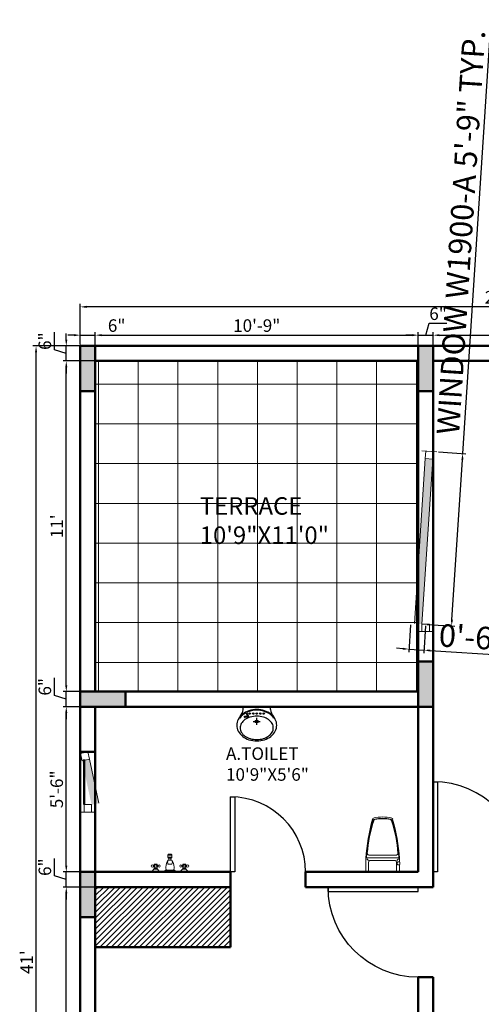
# Model space of a CAD drawing. Units: inches. Extents: x 3064 to 19385, y 846 to 15425.
# Tile 73 of 108: x 6445 to 6629, y 1725 to 2118. Entities that reach past the tile are written whole.
import ezdxf

# ---------------------------------------------------------------- set-up
doc = ezdxf.new("R2010")
doc.units = ezdxf.units.IN
for name, color, linetype, lineweight in [('A-ANNO-DIMS', 2, 'Continuous', 18), ('A-AREA-IDEN', 3, 'Continuous', 18), ('A-COLS', 1, 'Continuous', 35), ('A-DOOR', 3, 'Continuous', 25), ('A-FLOR-FIXT', 9, 'Continuous', 18), ('A-FLOR-PATT', 252, 'Continuous', 13), ('A-FURN-PATT', 252, 'Continuous', 13), ('A-GLAZ', 4, 'Continuous', 18), ('A-WALL', 7, 'Continuous', 50)]:
    doc.layers.add(name, color=color, linetype=linetype, lineweight=lineweight)
doc.layers.add('THIET-BI', color=21, linetype='Continuous')
doc.styles.get("Standard").update_dxf_attribs({"font": 'arial.ttf'})
doc.dimstyles.new('ISO-25', dxfattribs={"dimtxt": 9, "dimasz": 2.5, "dimexe": 1.25, "dimexo": 0.625, "dimtad": 1, "dimdec": 1, "dimlunit": 3, "dimtxsty": 'Standard', "dimcen": 2.5, "dimadec": 0, "dimazin": 0, "dimtfac": 1, "dimtdec": 1, "dimtmove": 0, "dimatfit": 3, "dimfxl": 1, "dimarcsym": 0})

# ---------------------------------------------------------------- blocks, each defined once
blk = doc.blocks.new('*U3')
for p, q in [((0, 0), (0, -6)), ((36, 0), (36, -6))]:
    blk.add_line(p, q)
blk.add_lwpolyline([(0, 0), (0, 36), (1.75, 36), (1.75, 0)], close=True)
blk.add_arc((0, 0), 36, 0, 90)
blk = doc.blocks.new('*U4')
for p, q in [((0, 0), (0, -6)), ((30, 0), (30, -6))]:
    blk.add_line(p, q)
blk.add_lwpolyline([(0, 0), (0, 30), (1.75, 30), (1.75, 0)], close=True)
blk.add_arc((0, 0), 30, 0, 90)
blk = doc.blocks.new('A$C430D11A0')
at = {"layer": 'THIET-BI'}
for p, q in [((90, 445), (90, 485)), ((475, 485), (90, 485)), ((475, 483), (90, 483)), ((475, 445), (475, 485)), ((129, 398), (158, 344)), ((138, 403), (176, 332)), ((282, 226), (282, 325)), ((233, 275), (332, 275))]:
    blk.add_line(p, q, dxfattribs=at)
for points in [[(565, 223, 0.121635), (545, 305, 0.10526), (482, 380, 0.088175), (393, 427, 0.079002), (282, 445, 0.079002), (172, 427, 0.088175), (83, 380, 0.10526), (20, 305, 0.121635), (0, 223, 0.121635), (20, 140, 0.10526), (83, 65, 0.088175), (172, 18, 0.079002), (282, 0, 0.079002), (393, 18, 0.088175), (482, 65, 0.10526), (545, 140, 0.121635)], [(517, 185, 0.134042), (501, 245, 0.106817), (449, 302, 0.082468), (376, 337, 0.070874), (282, 350, 0.070874), (189, 337, 0.082468), (116, 302, 0.106817), (64, 245, 0.134042), (47, 185, 0.134042), (64, 125, 0.106817), (116, 68, 0.082468), (189, 33, 0.070874), (282, 20, 0.070874), (376, 33, 0.082468), (449, 68, 0.106817), (501, 125, 0.134042)]]:
    blk.add_lwpolyline(points, format="xyb", close=True, dxfattribs=at)
for points in [[(523, 322, 0.07708), (476, 372, 0.088175), (390, 418, 0.079002), (282, 435, 0.079002), (175, 418, 0.035427), (138, 403, 0.07708)], [(129, 398, 0.043566), (89, 372, 0.07708), (42, 322, 0.041486)]]:
    blk.add_lwpolyline(points, format="xyb", dxfattribs=at)
for centre, radius in [((182, 388), 10.5), ((232, 388), 10.5), ((282, 275), 20), ((282, 275), 15), ((282, 388), 10.5), ((332, 388), 10.5), ((382, 388), 10.5)]:
    blk.add_circle(centre, radius, dxfattribs=at)
for centre, radius, start, end in [((-104, 469), 195, 320.8253, 352.9557), ((669, 469), 195, 187.0443, 219.1747), ((136, 285), 62.9, 69.643, 123.4774), ((136, 285), 52.9, 55.2455, 123.4774)]:
    blk.add_arc(centre, radius, start, end, dxfattribs=at)
blk = doc.blocks.new('WC-P05')
for p, q in [((-210, 430), (-210, 409)), ((-202, 532), (-202, 439)), ((-201, 439), (-180, 439)), ((-192, 542), (263, 542)), ((-171, 430), (-171, 409)), ((-163, 542), (-163, 401)), ((234, 542), (234, 401)), ((273, 532), (273, 352)), ((-202, 400), (-202, 352)), ((-201, 400), (-180, 400)), ((-192, 342), (263, 342)), ((-167, 379), (-188, 357)), ((-159, 303), (229, 303)), ((-143, 381), (214, 381)), ((237, 379), (258, 357))]:
    blk.add_line(p, q)
blk.add_lwpolyline([(-91, -222, 0.114547), (161, -222, 0.114547)], format="xyb")
for centre, radius, start, end in [((-201, 430), 9, 90, 180), ((-192, 532), 10, 90, 180), ((-180, 430), 9, 0, 90), ((263, 532), 10, 0, 90), ((-201, 409), 9, 180, 270), ((2309, 492), 2515, 183.2067, 196.1242), ((-192, 352), 10, 180, 270), ((1906, 447), 2103, 182.8743, 197.6554), ((-159, 280), 22.5, 90, 184.6246), ((-180, 409), 9, 270, 0), ((-143, 401), 20, 180, 270), ((-1836, 447), 2103, 342.3446, 357.1257), ((-2239, 492), 2515, 343.8727, 356.7933), ((214, 401), 20, 270, 0), ((229, 280), 22.5, 355.3754, 90), ((263, 352), 10, 270, 0), ((1906, 447), 2095, 184.6245, 197.5277), ((-1836, 447), 2095, 342.464, 355.3754), ((-86, -200), 22.5, 196.1242, 256.8994), ((-76, -184), 22.5, 197.6554, 257.5059), ((-70, -177), 22.5, 197.5277, 258.1005), ((35, 318), 536, 257.5059, 282.4941), ((36, 324), 535, 258.1005, 281.7373), ((140, -177), 22.5, 281.7373, 342.464), ((146, -184), 22.5, 282.4941, 342.3446), ((156, -200), 22.5, 283.0378, 343.8727)]:
    blk.add_arc(centre, radius, start, end)
blk = doc.blocks.new('Faucet - Bathroom front')
for p, q in [((-0.5, 4.25), (0.5, 4.25)), ((0.5, 3.75), (-0.5, 3.75)), ((-0.5, 3), (0.5, 3)), ((-0.25, 3), (-0.25, 3.5)), ((0.25, 3.5), (0.25, 3)), ((-5, 0), (-2.25, 0)), ((-4.5087, 0.25), (-2.7408, 0.25)), ((-4, 1.625), (-4.25, 1.625)), ((-4, 1.375), (-4.25, 1.375)), ((-3.1442, 0.75), (-4.0979, 0.75)), ((-3.25, 1.625), (-3, 1.625)), ((-3.25, 1.375), (-3, 1.375)), ((-1.5, 0), (1.5, 0)), ((-1, 0.5), (1, 0.5)), ((0.5, 2), (-0.5, 2)), ((2.25, 0), (5, 0)), ((2.7413, 0.25), (4.5092, 0.25)), ((3.25, 1.625), (3, 1.625)), ((3.25, 1.375), (3, 1.375)), ((4.1058, 0.75), (3.1521, 0.75)), ((4, 1.625), (4.25, 1.625)), ((4, 1.375), (4.25, 1.375))]:
    blk.add_line(p, q)
for points in [[(-0.5, 3.75), (-0.5, 4.25)], [(-0.25, 4.5), (0.25, 4.5)], [(0.25, 3.5), (-0.25, 3.5)], [(0.5, 4.25), (0.5, 3.75)]]:
    blk.add_lwpolyline(points)
for points in [[(-4, 1), (-4, 2), (-3.25, 2), (-3.25, 1)], [(3.25, 1), (3.25, 2), (4, 2), (4, 1)]]:
    blk.add_lwpolyline(points, close=True)
for centre in [(-4.5, 1.5), (-3.625, 1.5), (-2.75, 1.5), (2.75, 1.5), (3.625, 1.5), (4.5, 1.5)]:
    blk.add_circle(centre, 0.2795)
for centre, radius, start, end in [((3, 1), 4.0311, 150.2551, 187.125), ((0.6413, 2.5), 1.246, 156.3417, 203.6583), ((-0.2575, 4.2575), 0.2426, 88.22243, 181.7776), ((-0.2575, 3.7425), 0.2426, 178.2224, 271.7776), ((0.2575, 4.2575), 0.2426, 358.2224, 91.77757), ((0.2575, 3.7425), 0.2426, 268.2224, 1.777565), ((-3, 1), 4.0311, 352.875, 29.74488), ((-0.6413, 2.5), 1.246, 336.3417, 23.65835), ((-5.375, 1.375), 1.4252, 285.2551, 344.7449), ((-1.875, 1.375), 1.4252, 195.2551, 254.7449), ((-0.7962, -0.2038), 0.7327, 106.1502, 163.8498), ((0.7962, -0.2038), 0.7327, 16.1502, 73.84979), ((1.875, 1.375), 1.4252, 285.2551, 344.7449), ((5.375, 1.375), 1.4252, 195.2551, 254.7449)]:
    blk.add_arc(centre, radius, start, end)
blk = doc.blocks.new('*D372')
at = {"layer": 'A-ANNO-DIMS', "color": 0, "lineweight": -2, "transparency": 16777216}
for p, q in [((6474.41, 1771.99), (6462.18, 1771.99)), ((6463.43, 1576.49), (6463.43, 1769.49)), ((6474.41, 1573.99), (6462.18, 1573.99))]:
    blk.add_line(p, q, dxfattribs=at)
at = {"layer": 'A-ANNO-DIMS', "color": 0, "transparency": 16777216}
for points in [[(6463.02, 1769.49), (6463.85, 1769.49), (6463.43, 1771.99)], [(6463.02, 1576.49), (6463.85, 1576.49), (6463.43, 1573.99)]]:
    blk.add_solid(points, dxfattribs=at)
at = {"layer": 'Defpoints', "color": 0, "transparency": 16777216}
for p in [(6463.43, 1771.99), (6475.03, 1771.99), (6475.03, 1573.99)]:
    blk.add_point(p, dxfattribs=at)
at = {"layer": 'A-ANNO-DIMS', "color": 0, "transparency": 16777216, "insert": (6460.26, 1672.99), "char_height": 5, "attachment_point": 5, "rotation": 90}
blk.add_mtext('16\'-6"', dxfattribs=at)
blk = doc.blocks.new('*D373')
at = {"layer": 'A-ANNO-DIMS', "color": 0, "lineweight": -2, "transparency": 16777216}
for p, q in [((6458.69, 1776.41), (6458.69, 1783.44)), ((6463.43, 1780.49), (6463.43, 1782.99)), ((6474.41, 1777.99), (6462.18, 1777.99)), ((6463.43, 1771.99), (6463.43, 1777.99)), ((6463.43, 1771.99), (6463.43, 1777.99)), ((6463.43, 1774.99), (6458.69, 1776.41)), ((6474.41, 1771.99), (6462.18, 1771.99)), ((6463.43, 1769.49), (6463.43, 1766.99))]:
    blk.add_line(p, q, dxfattribs=at)
at = {"layer": 'A-ANNO-DIMS', "color": 0, "transparency": 16777216}
for points in [[(6463.02, 1780.49), (6463.85, 1780.49), (6463.43, 1777.99)], [(6463.02, 1769.49), (6463.85, 1769.49), (6463.43, 1771.99)]]:
    blk.add_solid(points, dxfattribs=at)
at = {"layer": 'Defpoints', "color": 0, "transparency": 16777216}
for p in [(6463.43, 1777.99), (6475.03, 1777.99), (6475.03, 1771.99)]:
    blk.add_point(p, dxfattribs=at)
at = {"layer": 'A-ANNO-DIMS', "color": 0, "transparency": 16777216, "insert": (6455.52, 1779.92), "char_height": 5, "attachment_point": 5, "rotation": 90}
blk.add_mtext('6"', dxfattribs=at)
blk = doc.blocks.new('*D374')
at = {"layer": 'A-ANNO-DIMS', "color": 0, "lineweight": -2, "transparency": 16777216}
for p, q in [((6468.41, 1843.99), (6462.18, 1843.99)), ((6463.43, 1780.49), (6463.43, 1841.49)), ((6474.41, 1777.99), (6462.18, 1777.99))]:
    blk.add_line(p, q, dxfattribs=at)
at = {"layer": 'A-ANNO-DIMS', "color": 0, "transparency": 16777216}
for points in [[(6463.02, 1841.49), (6463.85, 1841.49), (6463.43, 1843.99)], [(6463.02, 1780.49), (6463.85, 1780.49), (6463.43, 1777.99)]]:
    blk.add_solid(points, dxfattribs=at)
at = {"layer": 'Defpoints', "color": 0, "transparency": 16777216}
for p in [(6463.43, 1843.99), (6469.03, 1843.99), (6475.03, 1777.99)]:
    blk.add_point(p, dxfattribs=at)
at = {"layer": 'A-ANNO-DIMS', "color": 0, "transparency": 16777216, "insert": (6460.26, 1810.99), "char_height": 5, "attachment_point": 5, "rotation": 90}
blk.add_mtext('5\'-6"', dxfattribs=at)
blk = doc.blocks.new('*D367')
at = {"layer": 'A-ANNO-DIMS', "color": 0, "lineweight": -2, "transparency": 16777216}
for p, q in [((6458.69, 1848.41), (6458.69, 1855.44)), ((6463.43, 1852.49), (6463.43, 1854.99)), ((6463.43, 1846.99), (6458.69, 1848.41)), ((6468.41, 1849.99), (6462.18, 1849.99)), ((6463.43, 1843.99), (6463.43, 1849.99)), ((6463.43, 1843.99), (6463.43, 1849.99)), ((6468.41, 1843.99), (6462.18, 1843.99)), ((6463.43, 1841.49), (6463.43, 1838.99))]:
    blk.add_line(p, q, dxfattribs=at)
at = {"layer": 'A-ANNO-DIMS', "color": 0, "transparency": 16777216}
for points in [[(6463.02, 1852.49), (6463.85, 1852.49), (6463.43, 1849.99)], [(6463.02, 1841.49), (6463.85, 1841.49), (6463.43, 1843.99)]]:
    blk.add_solid(points, dxfattribs=at)
at = {"layer": 'Defpoints', "color": 0, "transparency": 16777216}
for p in [(6463.43, 1849.99), (6469.03, 1849.99), (6469.03, 1843.99)]:
    blk.add_point(p, dxfattribs=at)
at = {"layer": 'A-ANNO-DIMS', "color": 0, "transparency": 16777216, "insert": (6455.52, 1851.92), "char_height": 5, "attachment_point": 5, "rotation": 90}
blk.add_mtext('6"', dxfattribs=at)
blk = doc.blocks.new('*D368')
at = {"layer": 'A-ANNO-DIMS', "color": 0, "lineweight": -2, "transparency": 16777216}
for p, q in [((6474.41, 1981.99), (6462.18, 1981.99)), ((6463.43, 1852.49), (6463.43, 1979.49)), ((6468.41, 1849.99), (6462.18, 1849.99))]:
    blk.add_line(p, q, dxfattribs=at)
at = {"layer": 'A-ANNO-DIMS', "color": 0, "transparency": 16777216}
for points in [[(6463.02, 1979.49), (6463.85, 1979.49), (6463.43, 1981.99)], [(6463.02, 1852.49), (6463.85, 1852.49), (6463.43, 1849.99)]]:
    blk.add_solid(points, dxfattribs=at)
at = {"layer": 'Defpoints', "color": 0, "transparency": 16777216}
for p in [(6463.43, 1981.99), (6475.03, 1981.99), (6469.03, 1849.99)]:
    blk.add_point(p, dxfattribs=at)
at = {"layer": 'A-ANNO-DIMS', "color": 0, "transparency": 16777216, "insert": (6460.3, 1915.99), "char_height": 5, "attachment_point": 5, "rotation": 90}
blk.add_mtext("11'", dxfattribs=at)
blk = doc.blocks.new('*D369')
at = {"layer": 'A-ANNO-DIMS', "color": 0, "lineweight": -2, "transparency": 16777216}
for p, q in [((6458.69, 1986.41), (6458.69, 1993.44)), ((6463.43, 1990.49), (6463.43, 1992.99)), ((6463.43, 1984.99), (6458.69, 1986.41)), ((6474.41, 1987.99), (6462.18, 1987.99)), ((6463.43, 1981.99), (6463.43, 1987.99)), ((6463.43, 1981.99), (6463.43, 1987.99)), ((6474.41, 1981.99), (6462.18, 1981.99)), ((6463.43, 1979.49), (6463.43, 1976.99))]:
    blk.add_line(p, q, dxfattribs=at)
at = {"layer": 'A-ANNO-DIMS', "color": 0, "transparency": 16777216}
for points in [[(6463.02, 1990.49), (6463.85, 1990.49), (6463.43, 1987.99)], [(6463.02, 1979.49), (6463.85, 1979.49), (6463.43, 1981.99)]]:
    blk.add_solid(points, dxfattribs=at)
at = {"layer": 'Defpoints', "color": 0, "transparency": 16777216}
for p in [(6463.43, 1987.99), (6475.03, 1987.99), (6475.03, 1981.99)]:
    blk.add_point(p, dxfattribs=at)
at = {"layer": 'A-ANNO-DIMS', "color": 0, "transparency": 16777216, "insert": (6455.52, 1989.92), "char_height": 5, "attachment_point": 5, "rotation": 90}
blk.add_mtext('6"', dxfattribs=at)
blk = doc.blocks.new('*D370')
at = {"layer": 'A-ANNO-DIMS', "color": 0, "lineweight": -2, "transparency": 16777216}
for p, q in [((6468.41, 1987.99), (6450.1, 1987.99)), ((6451.35, 1498.49), (6451.35, 1985.49)), ((6468.41, 1495.99), (6450.1, 1495.99))]:
    blk.add_line(p, q, dxfattribs=at)
at = {"layer": 'A-ANNO-DIMS', "color": 0, "transparency": 16777216}
for points in [[(6450.94, 1985.49), (6451.77, 1985.49), (6451.35, 1987.99)], [(6450.94, 1498.49), (6451.77, 1498.49), (6451.35, 1495.99)]]:
    blk.add_solid(points, dxfattribs=at)
at = {"layer": 'Defpoints', "color": 0, "transparency": 16777216}
for p in [(6451.35, 1987.99), (6469.03, 1987.99), (6469.03, 1495.99)]:
    blk.add_point(p, dxfattribs=at)
at = {"layer": 'A-ANNO-DIMS', "color": 0, "transparency": 16777216, "insert": (6448.22, 1741.99), "char_height": 5, "attachment_point": 5, "rotation": 90}
blk.add_mtext("41'", dxfattribs=at)
blk = doc.blocks.new('*D341')
at = {"layer": 'A-ANNO-DIMS', "color": 0, "lineweight": -2, "transparency": 16777216}
for p, q in [((6469.03, 1988.61), (6469.03, 1993.55)), ((6475.03, 1988.61), (6475.03, 1993.55)), ((6466.53, 1992.3), (6464.03, 1992.3)), ((6469.03, 1992.3), (6475.03, 1992.3)), ((6477.53, 1992.3), (6487.06, 1992.3))]:
    blk.add_line(p, q, dxfattribs=at)
at = {"layer": 'A-ANNO-DIMS', "color": 0, "transparency": 16777216}
for points in [[(6466.53, 1992.72), (6466.53, 1991.88), (6469.03, 1992.3)], [(6477.53, 1992.72), (6477.53, 1991.88), (6475.03, 1992.3)]]:
    blk.add_solid(points, dxfattribs=at)
at = {"layer": 'Defpoints', "color": 0, "transparency": 16777216}
for p in [(6475.03, 1992.3), (6469.03, 1987.99), (6475.03, 1987.99)]:
    blk.add_point(p, dxfattribs=at)
at = {"layer": 'A-ANNO-DIMS', "color": 0, "transparency": 16777216, "insert": (6483.55, 1995.48), "char_height": 5, "attachment_point": 5}
blk.add_mtext('6"', dxfattribs=at)
blk = doc.blocks.new('*D349')
at = {"layer": 'A-ANNO-DIMS', "color": 0, "lineweight": -2, "transparency": 16777216}
for p, q in [((6475.03, 1988.61), (6475.03, 1993.55)), ((6604.03, 1988.61), (6604.03, 1993.55)), ((6477.53, 1992.3), (6601.53, 1992.3))]:
    blk.add_line(p, q, dxfattribs=at)
at = {"layer": 'A-ANNO-DIMS', "color": 0, "transparency": 16777216}
for points in [[(6477.53, 1992.72), (6477.53, 1991.88), (6475.03, 1992.3)], [(6601.53, 1992.72), (6601.53, 1991.88), (6604.03, 1992.3)]]:
    blk.add_solid(points, dxfattribs=at)
at = {"layer": 'Defpoints', "color": 0, "transparency": 16777216}
for p in [(6604.03, 1992.3), (6475.03, 1987.99), (6604.03, 1987.99)]:
    blk.add_point(p, dxfattribs=at)
at = {"layer": 'A-ANNO-DIMS', "color": 0, "transparency": 16777216, "insert": (6539.53, 1995.48), "char_height": 5, "attachment_point": 5}
blk.add_mtext('10\'-9"', dxfattribs=at)
blk = doc.blocks.new('*D343')
at = {"layer": 'A-ANNO-DIMS', "color": 0, "lineweight": -2, "transparency": 16777216}
for p, q in [((6607.03, 1992.3), (6608.46, 1997.04)), ((6608.46, 1997.04), (6615.48, 1997.04)), ((6604.03, 1988.61), (6604.03, 1993.55)), ((6610.03, 1988.61), (6610.03, 1993.55)), ((6601.53, 1992.3), (6599.03, 1992.3)), ((6604.03, 1992.3), (6610.03, 1992.3)), ((6604.03, 1992.3), (6610.03, 1992.3)), ((6612.53, 1992.3), (6615.03, 1992.3))]:
    blk.add_line(p, q, dxfattribs=at)
at = {"layer": 'A-ANNO-DIMS', "color": 0, "transparency": 16777216}
for points in [[(6601.53, 1992.72), (6601.53, 1991.88), (6604.03, 1992.3)], [(6612.53, 1992.72), (6612.53, 1991.88), (6610.03, 1992.3)]]:
    blk.add_solid(points, dxfattribs=at)
at = {"layer": 'Defpoints', "color": 0, "transparency": 16777216}
for p in [(6610.03, 1992.3), (6604.03, 1987.99), (6610.03, 1987.99)]:
    blk.add_point(p, dxfattribs=at)
at = {"layer": 'A-ANNO-DIMS', "color": 0, "transparency": 16777216, "insert": (6611.97, 2000.22), "char_height": 5, "attachment_point": 5}
blk.add_mtext('6"', dxfattribs=at)
blk = doc.blocks.new('*D344')
at = {"layer": 'A-ANNO-DIMS', "color": 0, "lineweight": -2, "transparency": 16777216}
for p, q in [((6610.03, 1988.61), (6610.03, 1993.55)), ((6805.03, 1988.61), (6805.03, 1993.55)), ((6612.53, 1992.3), (6802.53, 1992.3))]:
    blk.add_line(p, q, dxfattribs=at)
at = {"layer": 'A-ANNO-DIMS', "color": 0, "transparency": 16777216}
for points in [[(6612.53, 1992.72), (6612.53, 1991.88), (6610.03, 1992.3)], [(6802.53, 1992.72), (6802.53, 1991.88), (6805.03, 1992.3)]]:
    blk.add_solid(points, dxfattribs=at)
at = {"layer": 'Defpoints', "color": 0, "transparency": 16777216}
for p in [(6805.03, 1992.3), (6610.03, 1987.99), (6805.03, 1987.99)]:
    blk.add_point(p, dxfattribs=at)
at = {"layer": 'A-ANNO-DIMS', "color": 0, "transparency": 16777216, "insert": (6707.53, 1995.48), "char_height": 5, "attachment_point": 5}
blk.add_mtext('16\'-3"', dxfattribs=at)
blk = doc.blocks.new('*D340')
at = {"layer": 'A-ANNO-DIMS', "color": 0, "lineweight": -2, "transparency": 16777216}
for p, q in [((6469.03, 1988.61), (6469.03, 2004.85)), ((6811.03, 1988.61), (6811.03, 2004.85)), ((6808.53, 2003.6), (6471.53, 2003.6))]:
    blk.add_line(p, q, dxfattribs=at)
at = {"layer": 'A-ANNO-DIMS', "color": 0, "transparency": 16777216}
for points in [[(6471.53, 2004.02), (6471.53, 2003.18), (6469.03, 2003.6)], [(6808.53, 2004.02), (6808.53, 2003.18), (6811.03, 2003.6)]]:
    blk.add_solid(points, dxfattribs=at)
at = {"layer": 'Defpoints', "color": 0, "transparency": 16777216}
for p in [(6469.03, 2003.6), (6469.03, 1987.99), (6811.03, 1987.99)]:
    blk.add_point(p, dxfattribs=at)
at = {"layer": 'A-ANNO-DIMS', "color": 0, "transparency": 16777216, "insert": (6640.03, 2006.78), "char_height": 5, "attachment_point": 5}
blk.add_mtext('28\'-6"', dxfattribs=at)
blk = doc.blocks.new('WIN-600')
h = blk.add_hatch(color=256)
h.dxf.hatch_style = 1
h.paths.add_polyline_path([(3, 18), (0, 18), (0, 0), (3, 0)])
blk.add_line((3, 18), (3, 0))
blk.add_lwpolyline([(3, 18), (0, 18), (0, 21), (3, 21)], close=True)
blk = doc.blocks.new('WIN-1900-A')
h = blk.add_hatch(color=256)
h.dxf.hatch_style = 1
h.paths.add_polyline_path([(1.5, 0), (4.5, 0), (4.5, 66), (1.5, 66)])
for p, q in [((0, 69), (6, 69)), ((1.5, 66), (1.5, 0)), ((4.5, 66), (4.5, 0))]:
    blk.add_line(p, q)
blk.add_lwpolyline([(4.5, 66), (1.5, 66), (1.5, 69), (4.5, 69)], close=True)
blk = doc.blocks.new('*D433')
at = {"layer": 'A-ANNO-DIMS', "color": 0, "lineweight": -2, "transparency": 16777216}
for p, q in [((6621.84, 1945.07), (6633.12, 2118.25)), ((6612.14, 1945.71), (6623.09, 1944.99)), ((6617.52, 1878.71), (6621.68, 1942.58)), ((6607.65, 1876.85), (6618.61, 1876.14))]:
    blk.add_line(p, q, dxfattribs=at)
at = {"layer": 'A-ANNO-DIMS', "color": 0, "transparency": 16777216}
for points in [[(6621.26, 1942.61), (6622.09, 1942.55), (6621.84, 1945.07)], [(6617.11, 1878.74), (6617.94, 1878.69), (6617.36, 1876.22)]]:
    blk.add_solid(points, dxfattribs=at)
at = {"layer": 'Defpoints', "color": 0, "transparency": 16777216}
for p in [(6611.51, 1945.75), (6621.84, 1945.07), (6607.03, 1876.89)]:
    blk.add_point(p, dxfattribs=at)
at = {"layer": 'A-ANNO-DIMS', "color": 0, "transparency": 16777216, "insert": (6622.29, 2033.25), "char_height": 9, "attachment_point": 5, "rotation": 86.2748}
blk.add_mtext('WINDOW W1900-A 5\'-9" TYP.', dxfattribs=at)
blk = doc.blocks.new('*D434')
at = {"layer": 'A-ANNO-DIMS', "color": 0, "lineweight": -2, "transparency": 16777216}
for p, q in [((6601, 1876.66), (6600.29, 1865.71)), ((6606.99, 1876.27), (6606.28, 1865.32)), ((6597.88, 1867.12), (6595.38, 1867.28)), ((6600.37, 1866.95), (6606.36, 1866.56)), ((6608.85, 1866.4), (6667.34, 1862.59))]:
    blk.add_line(p, q, dxfattribs=at)
at = {"layer": 'A-ANNO-DIMS', "color": 0, "transparency": 16777216}
for points in [[(6597.9, 1867.53), (6597.85, 1866.7), (6600.37, 1866.95)], [(6608.88, 1866.82), (6608.83, 1865.99), (6606.36, 1866.56)]]:
    blk.add_solid(points, dxfattribs=at)
at = {"layer": 'Defpoints', "color": 0, "transparency": 16777216}
for p in [(6601.04, 1877.28), (6607.03, 1876.89), (6606.36, 1866.56)]:
    blk.add_point(p, dxfattribs=at)
at = {"layer": 'A-ANNO-DIMS', "color": 0, "transparency": 16777216, "insert": (6639.68, 1869.62), "char_height": 9, "attachment_point": 5, "rotation": 356.2748}
blk.add_mtext('0\'-6" TYP.', dxfattribs=at)

msp = doc.modelspace()

# ---------------------------------------------------------------- hatches: boundary and pattern name
at = {"layer": 'A-COLS'}
h = msp.add_hatch(color=256, dxfattribs=at)
h.dxf.hatch_style = 1
h.paths.add_polyline_path([(6469.03, 1969.99), (6475.03, 1969.99), (6475.03, 1987.99), (6469.03, 1987.99)])
h = msp.add_hatch(color=256, dxfattribs=at)
h.dxf.hatch_style = 1
h.paths.add_polyline_path([(6604.03, 1969.99), (6610.03, 1969.99), (6610.03, 1987.99), (6604.03, 1987.99)])
h = msp.add_hatch(color=256, dxfattribs=at)
h.dxf.hatch_style = 1
h.paths.add_polyline_path([(6604.03, 1843.99), (6610.03, 1843.99), (6610.03, 1861.99), (6604.03, 1861.99)])
h = msp.add_hatch(color=256, dxfattribs=at)
h.dxf.hatch_style = 1
h.paths.add_polyline_path([(6487.03, 1843.99), (6487.03, 1849.99), (6469.03, 1849.99), (6469.03, 1843.99)])
h = msp.add_hatch(color=256, dxfattribs=at)
h.dxf.hatch_style = 1
h.paths.add_polyline_path([(6469.03, 1759.99), (6475.03, 1759.99), (6475.03, 1777.99), (6469.03, 1777.99)])
at = {"layer": 'A-FLOR-PATT'}
h = msp.add_hatch(dxfattribs=at)
h.set_pattern_fill('ANSI37', color=256, scale=5, angle=45)
h.set_pattern_definition([(90, (2126.54, 591.649), (-15.875, 0), []), (180, (2126.54, 591.649), (-2e-15, -15.875), [])])
h.paths.add_polyline_path([(6475.03, 1981.99), (6475.03, 1969.99), (6475.03, 1849.99), (6604.03, 1849.99), (6604.03, 1861.99), (6604.03, 1981.99)])
at = {"layer": 'A-FURN-PATT'}
h = msp.add_hatch(dxfattribs=at)
h.set_pattern_fill('ANSI31', color=256, scale=0.5)
h.set_pattern_definition([(45, (2126.5405, 585.649), (-1.122532, 1.122532), [])])
h.paths.add_polyline_path([(6529.03, 1771.99), (6475.03, 1771.99), (6475.03, 1753.99), (6475.03, 1747.99), (6529.03, 1747.99)])

# ---------------------------------------------------------------- linework, layer by layer
at = {"layer": 'A-GLAZ'}
for p, q in [((6610.03, 1873.99), (6604.03, 1873.99)), ((6469.03, 1801.92), (6475.03, 1801.92))]:
    msp.add_line(p, q, dxfattribs=at)
for points in [[(6608.53, 1873.99), (6605.53, 1873.99), (6605.53, 1876.99), (6608.53, 1876.99)], [(6473.53, 1801.92), (6470.53, 1801.92), (6470.53, 1804.92), (6473.53, 1804.92)]]:
    msp.add_lwpolyline(points, close=True, dxfattribs=at)
at = {"layer": 'A-WALL'}
for p, q in [((6811.03, 1987.99), (6469.03, 1987.99)), ((6469.03, 1987.99), (6469.03, 1567.99)), ((6604.03, 1981.99), (6475.03, 1981.99)), ((6475.03, 1981.99), (6475.03, 1849.99)), ((6604.03, 1981.99), (6604.03, 1849.99)), ((6805.03, 1981.99), (6610.03, 1981.99)), ((6610.03, 1981.99), (6610.03, 1771.99)), ((6475.03, 1849.99), (6604.03, 1849.99)), ((6475.03, 1843.99), (6475.03, 1777.99)), ((6475.03, 1843.99), (6604.03, 1843.99)), ((6610.03, 1843.99), (6604.03, 1843.99)), ((6604.03, 1843.99), (6604.03, 1777.99)), ((6469.03, 1825.92), (6475.03, 1825.92)), ((6470.53, 1822.92), (6470.53, 1804.92)), ((6475.03, 1777.99), (6529.03, 1777.99)), ((6529.03, 1777.99), (6529.03, 1747.99)), ((6559.03, 1777.99), (6604.03, 1777.99)), ((6559.03, 1777.99), (6559.03, 1771.99)), ((6475.03, 1771.99), (6475.03, 1573.99)), ((6475.03, 1771.99), (6529.03, 1771.99)), ((6559.03, 1771.99), (6610.03, 1771.99)), ((6475.03, 1747.99), (6529.03, 1747.99)), ((6604.03, 1735.99), (6604.03, 1573.99)), ((6604.03, 1735.99), (6610.03, 1735.99)), ((6610.03, 1735.99), (6610.03, 1567.99))]:
    msp.add_line(p, q, dxfattribs=at)
for points in [[(6475.03, 1969.99), (6475.03, 1987.99), (6469.03, 1987.99), (6469.03, 1969.99)], [(6610.03, 1969.99), (6610.03, 1987.99), (6604.03, 1987.99), (6604.03, 1969.99)], [(6610.03, 1843.99), (6610.03, 1861.99), (6604.03, 1861.99), (6604.03, 1843.99)], [(6487.03, 1849.99), (6469.03, 1849.99), (6469.03, 1843.99), (6487.03, 1843.99)], [(6475.03, 1759.99), (6475.03, 1777.99), (6469.03, 1777.99), (6469.03, 1759.99)]]:
    msp.add_lwpolyline(points, close=True, dxfattribs=at)

# ---------------------------------------------------------------- block references
at = {"layer": 'A-DOOR'}
for name, p in [('*U3', (6610.03, 1777.99)), ('*U4', (6529.03, 1777.99))]:
    msp.add_blockref(name, p, dxfattribs=at)
at = {"layer": 'A-DOOR', "xscale": -1, "rotation": 90}
msp.add_blockref('*U3', (6604.03, 1771.99), dxfattribs=at)
at = {"layer": 'A-FLOR-FIXT'}
for name, p, xscale, yscale, zscale in [('A$C430D11A0', (6531.56, 1830.3), 0.0282220760332506, 0.0282220760332506, 0.0282220760332506), ('Faucet - Bathroom front', (6504.85, 1777.99), 1.573166238287219, 1.573166238287219, 1.573166238287219)]:
    msp.add_blockref(name, p, dxfattribs=dict(at, xscale=xscale, yscale=yscale, zscale=zscale))
at = {"layer": 'A-FLOR-FIXT', "xscale": 0.0282220760332506, "yscale": 0.0282220760332506, "zscale": 0.0282220760332506, "rotation": 180}
msp.add_blockref('WC-P05', (6590.81, 1793.28), dxfattribs=at)
at = {"layer": 'A-GLAZ'}
for name, p, rotation in [('WIN-1900-A', (6601.04, 1877.28), 356.2747581013879), ('WIN-600', (6473.54, 1804.82), 12.21571913413433)]:
    msp.add_blockref(name, p, dxfattribs=dict(at, rotation=rotation))

# ---------------------------------------------------------------- texts
at = {"layer": 'A-AREA-IDEN', "attachment_point": 1}
for s, insert, char_height in [('TERRACE\\P10\'9"X11\'0"', (6516.76, 1927.61), 7), ('A.TOILET\\P10\'9"X5\'6"', (6527.25, 1827.75), 5)]:
    msp.add_mtext_dynamic_manual_height_columns(s, width=67.5924, gutter_width=12.5, heights=[0], dxfattribs=dict(at, insert=insert, char_height=char_height))

# ---------------------------------------------------------------- dimensions: what is measured, and where the dimension line sits
at = {"layer": 'A-ANNO-DIMS'}
for base, p1, p2, angle, text, picture, middle in [((6621.84, 1945.07), (6607.03, 1876.89), (6611.51, 1945.75), 86.2748, 'WINDOW W1900-A <> TYP.', '*D433', (6622.29, 2033.25)), ((6606.36, 1866.56), (6601.04, 1877.28), (6607.03, 1876.89), 356.2748, '<> TYP.', '*D434', (6639.68, 1869.62))]:
    dim = msp.add_linear_dim(base=base, p1=p1, p2=p2, angle=angle, text=text, dimstyle='ISO-25', override={"dimdec": 1, "dimrnd": 0, "dimzin": 1, "dimlunit": 4, "dimfrac": 2}, dxfattribs=at)
    dim.commit()
    dim.dimension.update_dxf_attribs({"geometry": picture, "text_midpoint": middle})
for base, p1, p2, override, picture, middle in [((6469.03, 2003.6), (6811.03, 1987.99), (6469.03, 1987.99), {"dimtxt": 5, "dimclrd": 0, "dimclre": 0, "dimclrt": 0}, '*D340', (6640.03, 2006.78)), ((6610.03, 1992.3), (6604.03, 1987.99), (6610.03, 1987.99), {"dimtxt": 5, "dimclrd": 0, "dimclre": 0, "dimclrt": 0, "dimtmove": 1}, '*D343', (6609.08, 2000.22)), ((6475.03, 1992.3), (6469.03, 1987.99), (6475.03, 1987.99), {"dimtxt": 5, "dimclrd": 0, "dimclre": 0, "dimclrt": 0}, '*D341', (6483.55, 1995.48)), ((6604.03, 1992.3), (6475.03, 1987.99), (6604.03, 1987.99), {"dimtxt": 5, "dimclrd": 0, "dimclre": 0, "dimclrt": 0, "dimtmove": 1}, '*D349', (6539.53, 1995.48)), ((6805.03, 1992.3), (6610.03, 1987.99), (6805.03, 1987.99), {"dimtxt": 5, "dimclrd": 0, "dimclre": 0, "dimclrt": 0, "dimtmove": 1}, '*D344', (6707.53, 1995.48))]:
    dim = msp.add_linear_dim(base=base, p1=p1, p2=p2, dimstyle='ISO-25', override=override, dxfattribs=at)
    dim.commit()
    dim.dimension.update_dxf_attribs({"geometry": picture, "text_midpoint": middle})
for base, p1, p2, override, picture, middle in [((6463.43, 1987.99), (6475.03, 1981.99), (6475.03, 1987.99), {"dimtxt": 5, "dimclrd": 0, "dimclre": 0, "dimclrt": 0, "dimtmove": 1}, '*D369', (6455.52, 1987.04)), ((6451.35, 1987.99), (6469.03, 1495.99), (6469.03, 1987.99), {"dimtxt": 5, "dimclrd": 0, "dimclre": 0, "dimclrt": 0}, '*D370', (6448.22, 1741.99)), ((6463.43, 1981.99), (6469.03, 1849.99), (6475.03, 1981.99), {"dimtxt": 5, "dimclrd": 0, "dimclre": 0, "dimclrt": 0, "dimtmove": 1}, '*D368', (6460.3, 1915.99)), ((6463.43, 1849.99), (6469.03, 1843.99), (6469.03, 1849.99), {"dimtxt": 5, "dimclrd": 0, "dimclre": 0, "dimclrt": 0, "dimtmove": 1}, '*D367', (6455.52, 1849.04)), ((6463.43, 1843.99), (6475.03, 1777.99), (6469.03, 1843.99), {"dimtxt": 5, "dimclrd": 0, "dimclre": 0, "dimclrt": 0, "dimtmove": 1}, '*D374', (6460.26, 1810.99)), ((6463.43, 1777.99), (6475.03, 1771.99), (6475.03, 1777.99), {"dimtxt": 5, "dimclrd": 0, "dimclre": 0, "dimclrt": 0, "dimtmove": 1}, '*D373', (6455.52, 1777.04)), ((6463.43, 1771.99), (6475.03, 1573.99), (6475.03, 1771.99), {"dimtxt": 5, "dimclrd": 0, "dimclre": 0, "dimclrt": 0, "dimtmove": 1}, '*D372', (6460.26, 1672.99))]:
    dim = msp.add_linear_dim(base=base, p1=p1, p2=p2, angle=90, dimstyle='ISO-25', override=override, dxfattribs=at)
    dim.commit()
    dim.dimension.update_dxf_attribs({"geometry": picture, "text_midpoint": middle})

doc.saveas('drawing.dxf')
